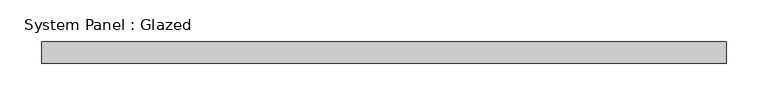
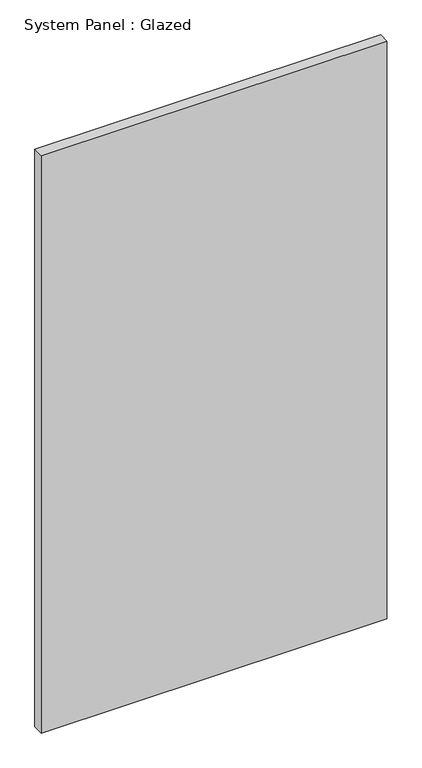
"""IFC4 building model written with IfcOpenShell, lengths in millimetres: plate geometry, System Panel : Glazed."""

from ifc_helpers import new_model, si_unit, origin, origin_with_axes, place, context, project, spatial, polyline, outline, extrude, source, transform, mapped, element, save


def system_panel_glazed_171f6735(model_context):
    return source(origin(), model_context, "Body", "SweptSolid", [
        extrude(outline(polyline([(409.575, 19.05), (-409.575, 19.05), (-409.575, 44.45), (409.575, 44.45), (409.575, 19.05)])), origin_with_axes(), (0.0, 0.0, 1.0), 1446.6725209),
    ])


if __name__ == "__main__":
    model = new_model("IFC4")
    model_context = context("Model", 3, world=origin())
    ifc_project = project(units=[si_unit("LENGTHUNIT", "METRE", prefix="MILLI")], contexts=[model_context])
    site = spatial("IfcSite", under=ifc_project)
    building = spatial("IfcBuilding", under=site)
    placement = place(None, origin())
    system_panel_glazed_shape = system_panel_glazed_171f6735(model_context)
    element("IfcPlate", 1, ObjectType="System Panel : Glazed", at=placement, inside=building, context=model_context, shape_type="MappedRepresentation", body=[
        mapped(system_panel_glazed_shape, transform((0.0, 0.0, 0.0), x_axis=(1.0, 0.0, 0.0), y_axis=(0.0, 1.0, 0.0), z_axis=(0.0, 0.0, 1.0))),
    ])
    save(model, "model.ifc")

# Revit data of these elements
# Type "System Panel : Glazed"
#   Construction Type Id = "GSP4R"
#   Analytic Construction = "1/8 in Pilkington single glazing"
#   Visual Light Transmittance = 0.9
#   Solar Heat Gain Coefficient = 0.86
#   Heat Transfer Coefficient (U) = 1.18115 BTU/(h·ft²·°F)
#   Define Thermal Properties by = 1
# Element 1 (IfcPlate, "System Panel : Glazed")
#   Materials on its faces: "Glass"
# Materials
#   "Glass": class "Glass", colour RGB 0 128 192, transparency 0.75, Description = "Soda Lime Glass", Cost = 0
